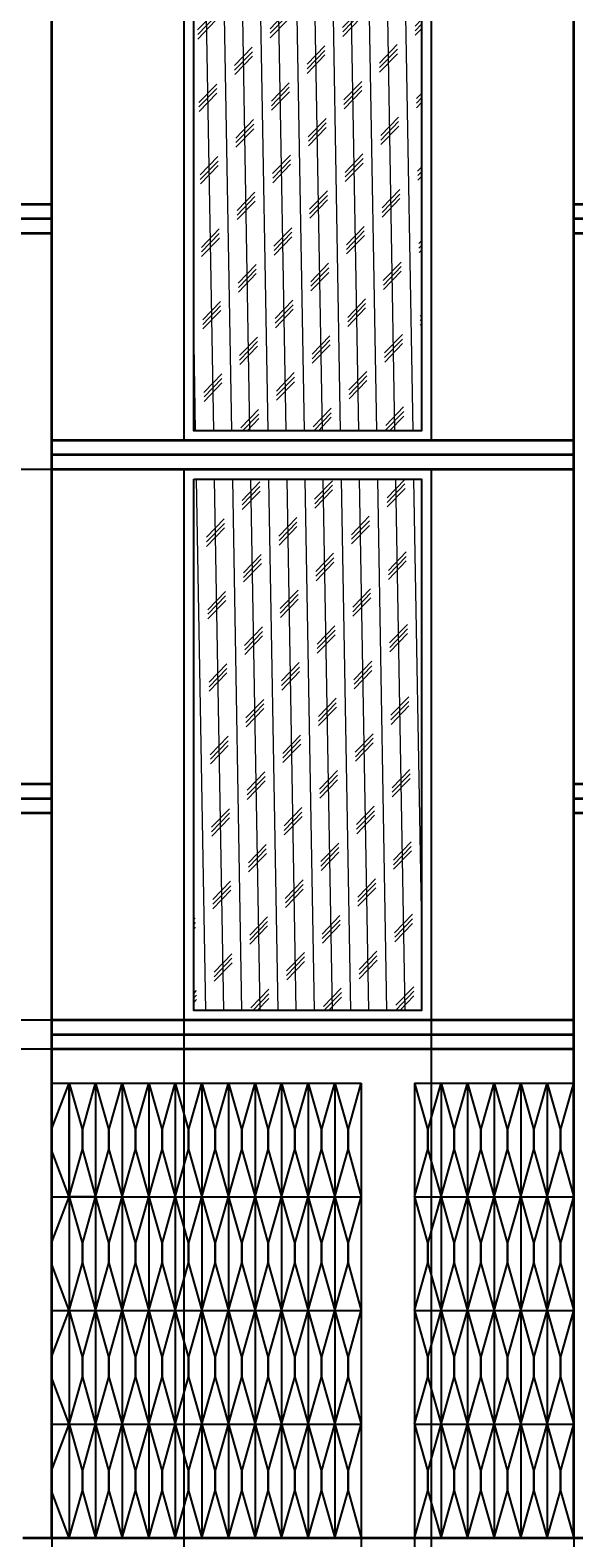
# Model space of a CAD drawing. Units: inches. Extents: x -742 to 1386, y -64 to 951.
# Tile 5 of 8: x 264 to 376, y 106 to 418. Entities that reach past the tile are written whole.
import ezdxf

# ---------------------------------------------------------------- set-up
doc = ezdxf.new("R2010")
doc.units = ezdxf.units.IN
doc.header["$MEASUREMENT"] = 0
for name, color, linetype, lineweight in [('A-ANNO-DIMS', 2, 'Continuous', 18), ('A-DOOR', 31, 'Continuous', 25), ('A-ELEV', 7, 'Continuous', 35), ('A-GLAZ', 4, 'Continuous', 25), ('A-GLAZ-PATT', 9, 'Continuous', 13)]:
    doc.layers.add(name, color=color, linetype=linetype, lineweight=lineweight)
doc.styles.get("Standard").update_dxf_attribs({"font": 'arial.ttf'})
doc.dimstyles.get("Standard").update_dxf_attribs({"dimtxt": 0.18, "dimasz": 0.18, "dimexe": 0.18, "dimexo": 0.0625, "dimgap": 0.09, "dimtad": 0, "dimtih": 1, "dimtoh": 1, "dimdec": 4, "dimzin": 0, "dimdsep": 46, "dimtxsty": 'Standard', "dimcen": 0.09, "dimadec": 0, "dimazin": 0, "dimtfac": 1, "dimtdec": 4, "dimtofl": 0, "dimtmove": 0, "dimatfit": 3, "dimfxl": 1, "dimtolj": 1, "dimtzin": 0, "dimarcsym": 0})
pattern_1 = [(91, (0, 0), (-3.74943, -0.065447), []), (226, (1.842, 1.907), (7.62975, -7.36796), [5.3033, -5.3033]), (226, (1.826, 2.845), (7.62975, -7.36796), [5.3033, -5.3033]), (226, (1.809, 3.782), (7.62975, -7.36796), [5.3033, -5.3033])]

# ---------------------------------------------------------------- blocks, each defined once
blk = doc.blocks.new('*D33')
at = {"layer": 'A-ANNO-DIMS', "color": 0, "lineweight": -2, "transparency": 16777216}
for p, q in [((268.23, 199.77), (268.23, -63.58)), ((332.25, 199.77), (332.25, -63.58)), ((268.41, -63.4), (299.84, -63.4)), ((332.07, -63.4), (300.63, -63.4))]:
    blk.add_line(p, q, dxfattribs=at)
at = {"layer": 'A-ANNO-DIMS', "color": 0, "transparency": 16777216}
for points in [[(268.41, -63.37), (268.41, -63.43), (268.23, -63.4)], [(332.07, -63.37), (332.07, -63.43), (332.25, -63.4)]]:
    blk.add_solid(points, dxfattribs=at)
at = {"layer": 'Defpoints', "color": 0, "transparency": 16777216}
for p in [(268.23, 199.83), (332.25, 199.83), (332.25, -63.4)]:
    blk.add_point(p, dxfattribs=at)
at = {"layer": 'A-ANNO-DIMS', "color": 0, "transparency": 16777216, "insert": (300.24, -63.4), "char_height": 0.18, "attachment_point": 5}
blk.add_mtext('\\A1;64.02', dxfattribs=at)
blk = doc.blocks.new('*D34')
at = {"layer": 'A-ANNO-DIMS', "color": 0, "lineweight": -2, "transparency": 16777216}
for p, q in [((332.25, 199.77), (332.25, -63.58)), ((343.24, 199.77), (343.24, -63.58)), ((332.43, -63.4), (337.29, -63.4)), ((343.06, -63.4), (338.2, -63.4))]:
    blk.add_line(p, q, dxfattribs=at)
at = {"layer": 'A-ANNO-DIMS', "color": 0, "transparency": 16777216}
for points in [[(332.43, -63.37), (332.43, -63.43), (332.25, -63.4)], [(343.06, -63.37), (343.06, -63.43), (343.24, -63.4)]]:
    blk.add_solid(points, dxfattribs=at)
at = {"layer": 'Defpoints', "color": 0, "transparency": 16777216}
for p in [(332.25, 199.83), (343.24, 199.83), (343.24, -63.4)]:
    blk.add_point(p, dxfattribs=at)
at = {"layer": 'A-ANNO-DIMS', "color": 0, "transparency": 16777216, "insert": (337.75, -63.4), "char_height": 0.18, "attachment_point": 5}
blk.add_mtext('\\A1;10.995', dxfattribs=at)
blk = doc.blocks.new('*D35')
at = {"layer": 'A-ANNO-DIMS', "color": 0, "lineweight": -2, "transparency": 16777216}
for p, q in [((343.24, 199.77), (343.24, -63.58)), ((376.23, 199.77), (376.23, -63.58)), ((343.42, -63.4), (359.27, -63.4)), ((376.05, -63.4), (360.2, -63.4))]:
    blk.add_line(p, q, dxfattribs=at)
at = {"layer": 'A-ANNO-DIMS', "color": 0, "transparency": 16777216}
for points in [[(343.42, -63.37), (343.42, -63.43), (343.24, -63.4)], [(376.05, -63.37), (376.05, -63.43), (376.23, -63.4)]]:
    blk.add_solid(points, dxfattribs=at)
at = {"layer": 'Defpoints', "color": 0, "transparency": 16777216}
for p in [(343.24, 199.83), (376.23, 199.83), (376.23, -63.4)]:
    blk.add_point(p, dxfattribs=at)
at = {"layer": 'A-ANNO-DIMS', "color": 0, "transparency": 16777216, "insert": (359.74, -63.4), "char_height": 0.18, "attachment_point": 5}
blk.add_mtext('\\A1;32.985', dxfattribs=at)
blk = doc.blocks.new('*D37')
at = {"layer": 'A-ANNO-DIMS', "color": 0, "lineweight": -2, "transparency": 16777216}
for p, q in [((268.23, 326.79), (268.23, -63.58)), ((295.56, 326.79), (295.56, -63.58)), ((268.41, -63.4), (281.43, -63.4)), ((295.38, -63.4), (282.36, -63.4))]:
    blk.add_line(p, q, dxfattribs=at)
at = {"layer": 'A-ANNO-DIMS', "color": 0, "transparency": 16777216}
for points in [[(268.41, -63.37), (268.41, -63.43), (268.23, -63.4)], [(295.38, -63.37), (295.38, -63.43), (295.56, -63.4)]]:
    blk.add_solid(points, dxfattribs=at)
at = {"layer": 'Defpoints', "color": 0, "transparency": 16777216}
for p in [(268.23, 326.85), (295.56, 326.85), (295.56, -63.4)]:
    blk.add_point(p, dxfattribs=at)
at = {"layer": 'A-ANNO-DIMS', "color": 0, "transparency": 16777216, "insert": (281.9, -63.4), "char_height": 0.18, "attachment_point": 5}
blk.add_mtext('\\A1;27.337', dxfattribs=at)
blk = doc.blocks.new('*D38')
at = {"layer": 'A-ANNO-DIMS', "color": 0, "lineweight": -2, "transparency": 16777216}
for p, q in [((295.56, 326.79), (295.56, -63.58)), ((346.7, 326.79), (346.7, -63.58)), ((295.74, -63.4), (320.74, -63.4)), ((346.52, -63.4), (321.52, -63.4))]:
    blk.add_line(p, q, dxfattribs=at)
at = {"layer": 'A-ANNO-DIMS', "color": 0, "transparency": 16777216}
for points in [[(295.74, -63.37), (295.74, -63.43), (295.56, -63.4)], [(346.52, -63.37), (346.52, -63.43), (346.7, -63.4)]]:
    blk.add_solid(points, dxfattribs=at)
at = {"layer": 'Defpoints', "color": 0, "transparency": 16777216}
for p in [(295.56, 326.85), (346.7, 326.85), (346.7, -63.4)]:
    blk.add_point(p, dxfattribs=at)
at = {"layer": 'A-ANNO-DIMS', "color": 0, "transparency": 16777216, "insert": (321.13, -63.4), "char_height": 0.18, "attachment_point": 5}
blk.add_mtext('\\A1;51.13', dxfattribs=at)
blk = doc.blocks.new('*D55')
at = {"layer": 'A-ANNO-DIMS', "color": 0, "lineweight": -2, "transparency": 16777216}
for p, q in [((295.5, 326.85), (-741.55, 326.85)), ((-741.37, 326.67), (-741.37, 270.04)), ((-741.37, 213.03), (-741.37, 269.67)), ((295.5, 212.85), (-741.55, 212.85))]:
    blk.add_line(p, q, dxfattribs=at)
at = {"layer": 'A-ANNO-DIMS', "color": 0, "transparency": 16777216}
for points in [[(-741.4, 326.67), (-741.34, 326.67), (-741.37, 326.85)], [(-741.4, 213.03), (-741.34, 213.03), (-741.37, 212.85)]]:
    blk.add_solid(points, dxfattribs=at)
at = {"layer": 'Defpoints', "color": 0, "transparency": 16777216}
for p in [(-741.37, 326.85), (295.56, 326.85), (295.56, 212.85)]:
    blk.add_point(p, dxfattribs=at)
at = {"layer": 'A-ANNO-DIMS', "color": 0, "transparency": 16777216, "insert": (-741.37, 269.85), "char_height": 0.18, "attachment_point": 5}
blk.add_mtext('\\A1;114', dxfattribs=at)
blk = doc.blocks.new('*D56')
at = {"layer": 'A-ANNO-DIMS', "color": 0, "lineweight": -2, "transparency": 16777216}
for p, q in [((268.17, 212.85), (-741.55, 212.85)), ((-741.37, 212.67), (-741.37, 210.04)), ((-741.37, 207.03), (-741.37, 209.67)), ((268.17, 206.85), (-741.55, 206.85))]:
    blk.add_line(p, q, dxfattribs=at)
at = {"layer": 'A-ANNO-DIMS', "color": 0, "transparency": 16777216}
for points in [[(-741.4, 212.67), (-741.34, 212.67), (-741.37, 212.85)], [(-741.4, 207.03), (-741.34, 207.03), (-741.37, 206.85)]]:
    blk.add_solid(points, dxfattribs=at)
at = {"layer": 'Defpoints', "color": 0, "transparency": 16777216}
for p in [(-741.37, 212.85), (268.23, 212.85), (268.23, 206.85)]:
    blk.add_point(p, dxfattribs=at)
at = {"layer": 'A-ANNO-DIMS', "color": 0, "transparency": 16777216, "insert": (-741.37, 209.85), "char_height": 0.18, "attachment_point": 5}
blk.add_mtext('\\A1;6', dxfattribs=at)

msp = doc.modelspace()

# ---------------------------------------------------------------- hatches: boundary and pattern name
at = {"layer": 'A-GLAZ-PATT', "transparency": 33554457}
h = msp.add_hatch(dxfattribs=at)
h.set_pattern_fill('CORK', color=256, scale=30, angle=91)
h.set_pattern_definition(pattern_1)
h.paths.add_polyline_path([(344.6973, 444.8548), (297.5643, 444.8548), (297.5643, 334.8548), (344.6973, 334.8548)])
h = msp.add_hatch(dxfattribs=at)
h.set_pattern_fill('CORK', color=256, scale=30, angle=91)
h.set_pattern_definition(pattern_1)
h.paths.add_polyline_path([(344.6973, 324.8548), (297.5643, 324.8548), (297.5643, 214.8548), (344.6973, 214.8548)])

# ---------------------------------------------------------------- linework, layer by layer
at = {"layer": 'A-DOOR'}
for p, q in [((268.2276, 199.8339), (332.2479, 199.8339)), ((268.2276, 190.4167), (271.776, 199.8339)), ((271.776, 199.8339), (271.776, 105.7399)), ((271.776, 199.8339), (274.5247, 190.0721)), ((274.5247, 190.0721), (277.2734, 199.8339)), ((277.2734, 199.8339), (277.2734, 105.7399)), ((277.2734, 199.8339), (280.0221, 190.0721)), ((280.0221, 190.0721), (282.7709, 199.8339)), ((282.7709, 199.8339), (282.7709, 105.7399)), ((282.7709, 199.8339), (285.5196, 190.0721)), ((285.5196, 190.0721), (288.2683, 199.8339)), ((288.2683, 199.8339), (288.2683, 105.7399)), ((288.2683, 199.8339), (291.017, 190.0721)), ((291.017, 190.0721), (293.7658, 199.8339)), ((293.7658, 199.8339), (293.7658, 105.7399)), ((293.7658, 199.8339), (296.5145, 190.0721)), ((296.5145, 190.0721), (299.2632, 199.8339)), ((299.2632, 199.8339), (299.2632, 105.7399)), ((299.2632, 199.8339), (302.012, 190.0721)), ((302.012, 190.0721), (304.7607, 199.8339)), ((304.7607, 199.8339), (304.7607, 105.7399)), ((304.7607, 199.8339), (307.5094, 190.0721)), ((307.5094, 190.0721), (310.2581, 199.8339)), ((310.2581, 199.8339), (310.2581, 105.7399)), ((310.2581, 199.8339), (313.0069, 190.0721)), ((313.0069, 190.0721), (315.7556, 199.8339)), ((315.7556, 199.8339), (315.7556, 105.7399)), ((315.7556, 199.8339), (318.5043, 190.0721)), ((318.5043, 190.0721), (321.253, 199.8339)), ((321.253, 199.8339), (321.253, 105.7399)), ((321.253, 199.8339), (324.0018, 190.0721)), ((324.0018, 190.0721), (326.7505, 199.8339)), ((326.7505, 199.8339), (326.7505, 105.7399)), ((326.7505, 199.8339), (329.4992, 190.0721)), ((329.4992, 190.0721), (332.2479, 199.8339)), ((332.2479, 199.8339), (332.2479, 105.7399)), ((343.2429, 199.8339), (343.2429, 105.7399)), ((343.2429, 199.8339), (345.9916, 190.0721)), ((343.2429, 199.8339), (376.2276, 199.8339)), ((345.9916, 190.0721), (348.7403, 199.8339)), ((348.7403, 199.8339), (348.7403, 105.7399)), ((348.7403, 199.8339), (351.489, 190.0721)), ((351.489, 190.0721), (354.2378, 199.8339)), ((354.2378, 199.8339), (354.2378, 105.7399)), ((354.2378, 199.8339), (356.9865, 190.0721)), ((356.9865, 190.0721), (359.7352, 199.8339)), ((359.7352, 199.8339), (359.7352, 105.7399)), ((359.7352, 199.8339), (362.4839, 190.0721)), ((362.4839, 190.0721), (365.2327, 199.8339)), ((365.2327, 199.8339), (365.2327, 105.7399)), ((365.2327, 199.8339), (367.9814, 190.0721)), ((367.9814, 190.0721), (370.7301, 199.8339)), ((370.7301, 199.8339), (370.7301, 105.7399)), ((370.7301, 199.8339), (373.4788, 190.0721)), ((373.4788, 190.0721), (376.2276, 199.8339)), ((376.2276, 199.8339), (376.2276, 105.7399)), ((274.5247, 186.0721), (274.5247, 190.0721)), ((274.5247, 190.0721), (274.5247, 186.0721)), ((280.0221, 186.0721), (280.0221, 190.0721)), ((280.0221, 190.0721), (280.0221, 186.0721)), ((285.5196, 186.0721), (285.5196, 190.0721)), ((285.5196, 190.0721), (285.5196, 186.0721)), ((291.017, 186.0721), (291.017, 190.0721)), ((291.017, 190.0721), (291.017, 186.0721)), ((296.5145, 186.0721), (296.5145, 190.0721)), ((296.5145, 190.0721), (296.5145, 186.0721)), ((302.012, 186.0721), (302.012, 190.0721)), ((302.012, 190.0721), (302.012, 186.0721)), ((307.5094, 186.0721), (307.5094, 190.0721)), ((307.5094, 190.0721), (307.5094, 186.0721)), ((313.0069, 186.0721), (313.0069, 190.0721)), ((313.0069, 190.0721), (313.0069, 186.0721)), ((318.5043, 186.0721), (318.5043, 190.0721)), ((318.5043, 190.0721), (318.5043, 186.0721)), ((324.0018, 186.0721), (324.0018, 190.0721)), ((324.0018, 190.0721), (324.0018, 186.0721)), ((329.4992, 186.0721), (329.4992, 190.0721)), ((329.4992, 190.0721), (329.4992, 186.0721)), ((345.9916, 186.0721), (345.9916, 190.0721)), ((345.9916, 190.0721), (345.9916, 186.0721)), ((351.489, 186.0721), (351.489, 190.0721)), ((351.489, 190.0721), (351.489, 186.0721)), ((356.9865, 186.0721), (356.9865, 190.0721)), ((356.9865, 190.0721), (356.9865, 186.0721)), ((362.4839, 186.0721), (362.4839, 190.0721)), ((362.4839, 190.0721), (362.4839, 186.0721)), ((367.9814, 186.0721), (367.9814, 190.0721)), ((367.9814, 190.0721), (367.9814, 186.0721)), ((373.4788, 186.0721), (373.4788, 190.0721)), ((373.4788, 190.0721), (373.4788, 186.0721)), ((271.776, 176.3104), (268.2276, 185.8171)), ((271.776, 176.3104), (274.5247, 186.0721)), ((274.5247, 186.0721), (277.2734, 176.3104)), ((277.2734, 176.3104), (280.0221, 186.0721)), ((280.0221, 186.0721), (282.7709, 176.3104)), ((282.7709, 176.3104), (285.5196, 186.0721)), ((285.5196, 186.0721), (288.2683, 176.3104)), ((288.2683, 176.3104), (291.017, 186.0721)), ((291.017, 186.0721), (293.7658, 176.3104)), ((293.7658, 176.3104), (296.5145, 186.0721)), ((296.5145, 186.0721), (299.2632, 176.3104)), ((299.2632, 176.3104), (302.012, 186.0721)), ((302.012, 186.0721), (304.7607, 176.3104)), ((304.7607, 176.3104), (307.5094, 186.0721)), ((307.5094, 186.0721), (310.2581, 176.3104)), ((310.2581, 176.3104), (313.0069, 186.0721)), ((313.0069, 186.0721), (315.7556, 176.3104)), ((315.7556, 176.3104), (318.5043, 186.0721)), ((318.5043, 186.0721), (321.253, 176.3104)), ((321.253, 176.3104), (324.0018, 186.0721)), ((324.0018, 186.0721), (326.7505, 176.3104)), ((326.7505, 176.3104), (329.4992, 186.0721)), ((329.4992, 186.0721), (332.2479, 176.3104)), ((343.2429, 176.3104), (345.9916, 186.0721)), ((345.9916, 186.0721), (348.7403, 176.3104)), ((348.7403, 176.3104), (351.489, 186.0721)), ((351.489, 186.0721), (354.2378, 176.3104)), ((354.2378, 176.3104), (356.9865, 186.0721)), ((356.9865, 186.0721), (359.7352, 176.3104)), ((359.7352, 176.3104), (362.4839, 186.0721)), ((362.4839, 186.0721), (365.2327, 176.3104)), ((365.2327, 176.3104), (367.9814, 186.0721)), ((367.9814, 186.0721), (370.7301, 176.3104)), ((370.7301, 176.3104), (373.4788, 186.0721)), ((373.4788, 186.0721), (376.2276, 176.3104)), ((268.2276, 176.3104), (332.2479, 176.3104)), ((268.2276, 166.8932), (271.776, 176.3104)), ((271.776, 176.3104), (274.5247, 166.5486)), ((274.5247, 166.5486), (277.2734, 176.3104)), ((277.2734, 176.3104), (280.0221, 166.5486)), ((280.0221, 166.5486), (282.7709, 176.3104)), ((282.7709, 176.3104), (285.5196, 166.5486)), ((285.5196, 166.5486), (288.2683, 176.3104)), ((288.2683, 176.3104), (291.017, 166.5486)), ((291.017, 166.5486), (293.7658, 176.3104)), ((293.7658, 176.3104), (296.5145, 166.5486)), ((296.5145, 166.5486), (299.2632, 176.3104)), ((299.2632, 176.3104), (302.012, 166.5486)), ((302.012, 166.5486), (304.7607, 176.3104)), ((304.7607, 176.3104), (307.5094, 166.5486)), ((307.5094, 166.5486), (310.2581, 176.3104)), ((310.2581, 176.3104), (313.0069, 166.5486)), ((313.0069, 166.5486), (315.7556, 176.3104)), ((315.7556, 176.3104), (318.5043, 166.5486)), ((318.5043, 166.5486), (321.253, 176.3104)), ((321.253, 176.3104), (324.0018, 166.5486)), ((324.0018, 166.5486), (326.7505, 176.3104)), ((326.7505, 176.3104), (329.4992, 166.5486)), ((329.4992, 166.5486), (332.2479, 176.3104)), ((343.2429, 176.3104), (345.9916, 166.5486)), ((343.2429, 176.3104), (376.2276, 176.3104)), ((345.9916, 166.5486), (348.7403, 176.3104)), ((348.7403, 176.3104), (351.489, 166.5486)), ((351.489, 166.5486), (354.2378, 176.3104)), ((354.2378, 176.3104), (356.9865, 166.5486)), ((356.9865, 166.5486), (359.7352, 176.3104)), ((359.7352, 176.3104), (362.4839, 166.5486)), ((362.4839, 166.5486), (365.2327, 176.3104)), ((365.2327, 176.3104), (367.9814, 166.5486)), ((367.9814, 166.5486), (370.7301, 176.3104)), ((370.7301, 176.3104), (373.4788, 166.5486)), ((373.4788, 166.5486), (376.2276, 176.3104)), ((274.5247, 162.5486), (274.5247, 166.5486)), ((274.5247, 166.5486), (274.5247, 162.5486)), ((280.0221, 162.5486), (280.0221, 166.5486)), ((280.0221, 166.5486), (280.0221, 162.5486)), ((285.5196, 162.5486), (285.5196, 166.5486)), ((285.5196, 166.5486), (285.5196, 162.5486)), ((291.017, 162.5486), (291.017, 166.5486)), ((291.017, 166.5486), (291.017, 162.5486)), ((296.5145, 162.5486), (296.5145, 166.5486)), ((296.5145, 166.5486), (296.5145, 162.5486)), ((302.012, 162.5486), (302.012, 166.5486)), ((302.012, 166.5486), (302.012, 162.5486)), ((307.5094, 162.5486), (307.5094, 166.5486)), ((307.5094, 166.5486), (307.5094, 162.5486)), ((313.0069, 162.5486), (313.0069, 166.5486)), ((313.0069, 166.5486), (313.0069, 162.5486)), ((318.5043, 162.5486), (318.5043, 166.5486)), ((318.5043, 166.5486), (318.5043, 162.5486)), ((324.0018, 162.5486), (324.0018, 166.5486)), ((324.0018, 166.5486), (324.0018, 162.5486)), ((329.4992, 162.5486), (329.4992, 166.5486)), ((329.4992, 166.5486), (329.4992, 162.5486)), ((345.9916, 162.5486), (345.9916, 166.5486)), ((345.9916, 166.5486), (345.9916, 162.5486)), ((351.489, 162.5486), (351.489, 166.5486)), ((351.489, 166.5486), (351.489, 162.5486)), ((356.9865, 162.5486), (356.9865, 166.5486)), ((356.9865, 166.5486), (356.9865, 162.5486)), ((362.4839, 162.5486), (362.4839, 166.5486)), ((362.4839, 166.5486), (362.4839, 162.5486)), ((367.9814, 162.5486), (367.9814, 166.5486)), ((367.9814, 166.5486), (367.9814, 162.5486)), ((373.4788, 162.5486), (373.4788, 166.5486)), ((373.4788, 166.5486), (373.4788, 162.5486)), ((271.776, 152.7869), (268.2276, 162.2936)), ((271.776, 152.7869), (274.5247, 162.5486)), ((274.5247, 162.5486), (277.2734, 152.7869)), ((277.2734, 152.7869), (280.0221, 162.5486)), ((280.0221, 162.5486), (282.7709, 152.7869)), ((282.7709, 152.7869), (285.5196, 162.5486)), ((285.5196, 162.5486), (288.2683, 152.7869)), ((288.2683, 152.7869), (291.017, 162.5486)), ((291.017, 162.5486), (293.7658, 152.7869)), ((293.7658, 152.7869), (296.5145, 162.5486)), ((296.5145, 162.5486), (299.2632, 152.7869)), ((299.2632, 152.7869), (302.012, 162.5486)), ((302.012, 162.5486), (304.7607, 152.7869)), ((304.7607, 152.7869), (307.5094, 162.5486)), ((307.5094, 162.5486), (310.2581, 152.7869)), ((310.2581, 152.7869), (313.0069, 162.5486)), ((313.0069, 162.5486), (315.7556, 152.7869)), ((315.7556, 152.7869), (318.5043, 162.5486)), ((318.5043, 162.5486), (321.253, 152.7869)), ((321.253, 152.7869), (324.0018, 162.5486)), ((324.0018, 162.5486), (326.7505, 152.7869)), ((326.7505, 152.7869), (329.4992, 162.5486)), ((329.4992, 162.5486), (332.2479, 152.7869)), ((343.2429, 152.7869), (345.9916, 162.5486)), ((345.9916, 162.5486), (348.7403, 152.7869)), ((348.7403, 152.7869), (351.489, 162.5486)), ((351.489, 162.5486), (354.2378, 152.7869)), ((354.2378, 152.7869), (356.9865, 162.5486)), ((356.9865, 162.5486), (359.7352, 152.7869)), ((359.7352, 152.7869), (362.4839, 162.5486)), ((362.4839, 162.5486), (365.2327, 152.7869)), ((365.2327, 152.7869), (367.9814, 162.5486)), ((367.9814, 162.5486), (370.7301, 152.7869)), ((370.7301, 152.7869), (373.4788, 162.5486)), ((373.4788, 162.5486), (376.2276, 152.7869)), ((268.2276, 152.7869), (332.2479, 152.7869)), ((268.2276, 143.3697), (271.776, 152.7869)), ((271.776, 152.7869), (274.5247, 143.0251)), ((274.5247, 143.0251), (277.2734, 152.7869)), ((277.2734, 152.7869), (280.0221, 143.0251)), ((280.0221, 143.0251), (282.7709, 152.7869)), ((282.7709, 152.7869), (285.5196, 143.0251)), ((285.5196, 143.0251), (288.2683, 152.7869)), ((288.2683, 152.7869), (291.017, 143.0251)), ((291.017, 143.0251), (293.7658, 152.7869)), ((293.7658, 152.7869), (296.5145, 143.0251)), ((296.5145, 143.0251), (299.2632, 152.7869)), ((299.2632, 152.7869), (302.012, 143.0251)), ((302.012, 143.0251), (304.7607, 152.7869)), ((304.7607, 152.7869), (307.5094, 143.0251)), ((307.5094, 143.0251), (310.2581, 152.7869)), ((310.2581, 152.7869), (313.0069, 143.0251)), ((313.0069, 143.0251), (315.7556, 152.7869)), ((315.7556, 152.7869), (318.5043, 143.0251)), ((318.5043, 143.0251), (321.253, 152.7869)), ((321.253, 152.7869), (324.0018, 143.0251)), ((324.0018, 143.0251), (326.7505, 152.7869)), ((326.7505, 152.7869), (329.4992, 143.0251)), ((329.4992, 143.0251), (332.2479, 152.7869)), ((343.2429, 152.7869), (345.9916, 143.0251)), ((343.2429, 152.7869), (376.2276, 152.7869)), ((345.9916, 143.0251), (348.7403, 152.7869)), ((348.7403, 152.7869), (351.489, 143.0251)), ((351.489, 143.0251), (354.2378, 152.7869)), ((354.2378, 152.7869), (356.9865, 143.0251)), ((356.9865, 143.0251), (359.7352, 152.7869)), ((359.7352, 152.7869), (362.4839, 143.0251)), ((362.4839, 143.0251), (365.2327, 152.7869)), ((365.2327, 152.7869), (367.9814, 143.0251)), ((367.9814, 143.0251), (370.7301, 152.7869)), ((370.7301, 152.7869), (373.4788, 143.0251)), ((373.4788, 143.0251), (376.2276, 152.7869)), ((274.5247, 139.0251), (274.5247, 143.0251)), ((274.5247, 143.0251), (274.5247, 139.0251)), ((280.0221, 139.0251), (280.0221, 143.0251)), ((280.0221, 143.0251), (280.0221, 139.0251)), ((285.5196, 139.0251), (285.5196, 143.0251)), ((285.5196, 143.0251), (285.5196, 139.0251)), ((291.017, 139.0251), (291.017, 143.0251)), ((291.017, 143.0251), (291.017, 139.0251)), ((296.5145, 139.0251), (296.5145, 143.0251)), ((296.5145, 143.0251), (296.5145, 139.0251)), ((302.012, 139.0251), (302.012, 143.0251)), ((302.012, 143.0251), (302.012, 139.0251)), ((307.5094, 139.0251), (307.5094, 143.0251)), ((307.5094, 143.0251), (307.5094, 139.0251)), ((313.0069, 139.0251), (313.0069, 143.0251)), ((313.0069, 143.0251), (313.0069, 139.0251)), ((318.5043, 139.0251), (318.5043, 143.0251)), ((318.5043, 143.0251), (318.5043, 139.0251)), ((324.0018, 139.0251), (324.0018, 143.0251)), ((324.0018, 143.0251), (324.0018, 139.0251)), ((329.4992, 139.0251), (329.4992, 143.0251)), ((329.4992, 143.0251), (329.4992, 139.0251)), ((345.9916, 139.0251), (345.9916, 143.0251)), ((345.9916, 143.0251), (345.9916, 139.0251)), ((351.489, 139.0251), (351.489, 143.0251)), ((351.489, 143.0251), (351.489, 139.0251)), ((356.9865, 139.0251), (356.9865, 143.0251)), ((356.9865, 143.0251), (356.9865, 139.0251)), ((362.4839, 139.0251), (362.4839, 143.0251)), ((362.4839, 143.0251), (362.4839, 139.0251)), ((367.9814, 139.0251), (367.9814, 143.0251)), ((367.9814, 143.0251), (367.9814, 139.0251)), ((373.4788, 139.0251), (373.4788, 143.0251)), ((373.4788, 143.0251), (373.4788, 139.0251)), ((271.776, 129.2634), (268.2276, 138.7701)), ((271.776, 129.2634), (274.5247, 139.0251)), ((274.5247, 139.0251), (277.2734, 129.2634)), ((277.2734, 129.2634), (280.0221, 139.0251)), ((280.0221, 139.0251), (282.7709, 129.2634)), ((282.7709, 129.2634), (285.5196, 139.0251)), ((285.5196, 139.0251), (288.2683, 129.2634)), ((288.2683, 129.2634), (291.017, 139.0251)), ((291.017, 139.0251), (293.7658, 129.2634)), ((293.7658, 129.2634), (296.5145, 139.0251)), ((296.5145, 139.0251), (299.2632, 129.2634)), ((299.2632, 129.2634), (302.012, 139.0251)), ((302.012, 139.0251), (304.7607, 129.2634)), ((304.7607, 129.2634), (307.5094, 139.0251)), ((307.5094, 139.0251), (310.2581, 129.2634)), ((310.2581, 129.2634), (313.0069, 139.0251)), ((313.0069, 139.0251), (315.7556, 129.2634)), ((315.7556, 129.2634), (318.5043, 139.0251)), ((318.5043, 139.0251), (321.253, 129.2634)), ((321.253, 129.2634), (324.0018, 139.0251)), ((324.0018, 139.0251), (326.7505, 129.2634)), ((326.7505, 129.2634), (329.4992, 139.0251)), ((329.4992, 139.0251), (332.2479, 129.2634)), ((343.2429, 129.2634), (345.9916, 139.0251)), ((345.9916, 139.0251), (348.7403, 129.2634)), ((348.7403, 129.2634), (351.489, 139.0251)), ((351.489, 139.0251), (354.2378, 129.2634)), ((354.2378, 129.2634), (356.9865, 139.0251)), ((356.9865, 139.0251), (359.7352, 129.2634)), ((359.7352, 129.2634), (362.4839, 139.0251)), ((362.4839, 139.0251), (365.2327, 129.2634)), ((365.2327, 129.2634), (367.9814, 139.0251)), ((367.9814, 139.0251), (370.7301, 129.2634)), ((370.7301, 129.2634), (373.4788, 139.0251)), ((373.4788, 139.0251), (376.2276, 129.2634)), ((268.2276, 129.2634), (332.2479, 129.2634)), ((268.2276, 119.8462), (271.776, 129.2634)), ((271.776, 129.2634), (274.5247, 119.5016)), ((274.5247, 119.5016), (277.2734, 129.2634)), ((277.2734, 129.2634), (280.0221, 119.5016)), ((280.0221, 119.5016), (282.7709, 129.2634)), ((282.7709, 129.2634), (285.5196, 119.5016)), ((285.5196, 119.5016), (288.2683, 129.2634)), ((288.2683, 129.2634), (291.017, 119.5016)), ((291.017, 119.5016), (293.7658, 129.2634)), ((293.7658, 129.2634), (296.5145, 119.5016)), ((296.5145, 119.5016), (299.2632, 129.2634)), ((299.2632, 129.2634), (302.012, 119.5016)), ((302.012, 119.5016), (304.7607, 129.2634)), ((304.7607, 129.2634), (307.5094, 119.5016)), ((307.5094, 119.5016), (310.2581, 129.2634)), ((310.2581, 129.2634), (313.0069, 119.5016)), ((313.0069, 119.5016), (315.7556, 129.2634)), ((315.7556, 129.2634), (318.5043, 119.5016)), ((318.5043, 119.5016), (321.253, 129.2634)), ((321.253, 129.2634), (324.0018, 119.5016)), ((324.0018, 119.5016), (326.7505, 129.2634)), ((326.7505, 129.2634), (329.4992, 119.5016)), ((329.4992, 119.5016), (332.2479, 129.2634)), ((343.2429, 129.2634), (345.9916, 119.5016)), ((343.2429, 129.2634), (376.2276, 129.2634)), ((345.9916, 119.5016), (348.7403, 129.2634)), ((348.7403, 129.2634), (351.489, 119.5016)), ((351.489, 119.5016), (354.2378, 129.2634)), ((354.2378, 129.2634), (356.9865, 119.5016)), ((356.9865, 119.5016), (359.7352, 129.2634)), ((359.7352, 129.2634), (362.4839, 119.5016)), ((362.4839, 119.5016), (365.2327, 129.2634)), ((365.2327, 129.2634), (367.9814, 119.5016)), ((367.9814, 119.5016), (370.7301, 129.2634)), ((370.7301, 129.2634), (373.4788, 119.5016)), ((373.4788, 119.5016), (376.2276, 129.2634)), ((274.5247, 115.5016), (274.5247, 119.5016)), ((274.5247, 119.5016), (274.5247, 115.5016)), ((280.0221, 115.5016), (280.0221, 119.5016)), ((280.0221, 119.5016), (280.0221, 115.5016)), ((285.5196, 115.5016), (285.5196, 119.5016)), ((285.5196, 119.5016), (285.5196, 115.5016)), ((291.017, 115.5016), (291.017, 119.5016)), ((291.017, 119.5016), (291.017, 115.5016)), ((296.5145, 115.5016), (296.5145, 119.5016)), ((296.5145, 119.5016), (296.5145, 115.5016)), ((302.012, 115.5016), (302.012, 119.5016)), ((302.012, 119.5016), (302.012, 115.5016)), ((307.5094, 115.5016), (307.5094, 119.5016)), ((307.5094, 119.5016), (307.5094, 115.5016)), ((313.0069, 115.5016), (313.0069, 119.5016)), ((313.0069, 119.5016), (313.0069, 115.5016)), ((318.5043, 115.5016), (318.5043, 119.5016)), ((318.5043, 119.5016), (318.5043, 115.5016)), ((324.0018, 115.5016), (324.0018, 119.5016)), ((324.0018, 119.5016), (324.0018, 115.5016)), ((329.4992, 115.5016), (329.4992, 119.5016)), ((329.4992, 119.5016), (329.4992, 115.5016)), ((345.9916, 115.5016), (345.9916, 119.5016)), ((345.9916, 119.5016), (345.9916, 115.5016)), ((351.489, 115.5016), (351.489, 119.5016)), ((351.489, 119.5016), (351.489, 115.5016)), ((356.9865, 115.5016), (356.9865, 119.5016)), ((356.9865, 119.5016), (356.9865, 115.5016)), ((362.4839, 115.5016), (362.4839, 119.5016)), ((362.4839, 119.5016), (362.4839, 115.5016)), ((367.9814, 115.5016), (367.9814, 119.5016)), ((367.9814, 119.5016), (367.9814, 115.5016)), ((373.4788, 115.5016), (373.4788, 119.5016)), ((373.4788, 119.5016), (373.4788, 115.5016)), ((271.776, 105.7399), (274.5247, 115.5016)), ((274.5247, 115.5016), (277.2734, 105.7399)), ((277.2734, 105.7399), (280.0221, 115.5016)), ((280.0221, 115.5016), (282.7709, 105.7399)), ((282.7709, 105.7399), (285.5196, 115.5016)), ((285.5196, 115.5016), (288.2683, 105.7399)), ((288.2683, 105.7399), (291.017, 115.5016)), ((291.017, 115.5016), (293.7658, 105.7399)), ((293.7658, 105.7399), (296.5145, 115.5016)), ((296.5145, 115.5016), (299.2632, 105.7399)), ((299.2632, 105.7399), (302.012, 115.5016)), ((302.012, 115.5016), (304.7607, 105.7399)), ((304.7607, 105.7399), (307.5094, 115.5016)), ((307.5094, 115.5016), (310.2581, 105.7399)), ((310.2581, 105.7399), (313.0069, 115.5016)), ((313.0069, 115.5016), (315.7556, 105.7399)), ((315.7556, 105.7399), (318.5043, 115.5016)), ((318.5043, 115.5016), (321.253, 105.7399)), ((321.253, 105.7399), (324.0018, 115.5016)), ((324.0018, 115.5016), (326.7505, 105.7399)), ((326.7505, 105.7399), (329.4992, 115.5016)), ((329.4992, 115.5016), (332.2479, 105.7399)), ((343.2429, 105.7399), (345.9916, 115.5016)), ((345.9916, 115.5016), (348.7403, 105.7399)), ((348.7403, 105.7399), (351.489, 115.5016)), ((351.489, 115.5016), (354.2378, 105.7399)), ((354.2378, 105.7399), (356.9865, 115.5016)), ((356.9865, 115.5016), (359.7352, 105.7399)), ((359.7352, 105.7399), (362.4839, 115.5016)), ((362.4839, 115.5016), (365.2327, 105.7399)), ((365.2327, 105.7399), (367.9814, 115.5016)), ((367.9814, 115.5016), (370.7301, 105.7399)), ((370.7301, 105.7399), (373.4788, 115.5016)), ((373.4788, 115.5016), (376.2276, 105.7399)), ((271.776, 105.7399), (268.2276, 115.2466)), ((268.2276, 105.7399), (376.2276, 105.7399))]:
    msp.add_line(p, q, dxfattribs=at)
msp.add_lwpolyline([(271.776, 199.8339), (277.2734, 199.8339), (277.2734, 176.3104), (271.776, 176.3104)], close=True, dxfattribs=at)
at = {"layer": 'A-ELEV'}
for p, q in [((268.2276, 105.7399), (268.2276, 835.7799)), ((376.2276, 105.7399), (376.2276, 835.7799)), ((-37.7724, 381.7399), (268.2276, 381.7399)), ((376.2276, 381.7399), (682.2276, 381.7399)), ((-37.7724, 378.7399), (268.2276, 378.7399)), ((376.2276, 378.7399), (682.2276, 378.7399)), ((-37.7724, 375.7399), (268.2276, 375.7399)), ((376.2276, 375.7399), (682.2276, 375.7399)), ((376.2276, 332.8548), (268.2276, 332.8548)), ((376.2276, 329.8548), (268.2276, 329.8548)), ((376.2276, 326.8548), (268.2276, 326.8548)), ((-37.7724, 261.7399), (268.2276, 261.7399)), ((376.2276, 261.7399), (622.2276, 261.7399)), ((-37.7724, 258.7399), (268.2276, 258.7399)), ((376.2276, 258.7399), (622.2276, 258.7399)), ((-37.7724, 255.7399), (268.2276, 255.7399)), ((376.2276, 255.7399), (622.2276, 255.7399)), ((376.2276, 212.8548), (268.2276, 212.8548)), ((376.2276, 209.8548), (268.2276, 209.8548)), ((376.2276, 206.8548), (268.2276, 206.8548)), ((262.2276, 105.7399), (682.2276, 105.7399))]:
    msp.add_line(p, q, dxfattribs=at)
at = {"layer": 'A-GLAZ'}
for points in [[(295.5643, 446.8548), (346.6973, 446.8548), (346.6973, 332.8548), (295.5643, 332.8548)], [(297.5643, 444.8548), (344.6973, 444.8548), (344.6973, 334.8548), (297.5643, 334.8548)], [(295.5643, 326.8548), (346.6973, 326.8548), (346.6973, 212.8548), (295.5643, 212.8548)], [(297.5643, 324.8548), (344.6973, 324.8548), (344.6973, 214.8548), (297.5643, 214.8548)]]:
    msp.add_lwpolyline(points, close=True, dxfattribs=at)

# ---------------------------------------------------------------- dimensions: what is measured, and where the dimension line sits
at = {"layer": 'A-ANNO-DIMS'}
for base, p1, p2, picture, middle in [((-741.3711, 326.8548), (295.5643, 212.8548), (295.5643, 326.8548), '*D55', (-741.3711, 269.8548)), ((-741.3711, 212.8548), (268.2276, 206.8548), (268.2276, 212.8548), '*D56', (-741.3711, 209.8548))]:
    dim = msp.add_linear_dim(base=base, p1=p1, p2=p2, angle=90, dimstyle='Standard', override={"dimdec": 0, "dimlfac": 1, "dimrnd": 0, "dimzin": 0, "dimdsep": 46, "dimlunit": 2}, dxfattribs=at)
    dim.commit()
    dim.dimension.update_dxf_attribs({"geometry": picture, "text_midpoint": middle})
for base, p1, p2, override, picture, middle in [((295.5643, -63.3971), (268.2276, 326.8548), (295.5643, 326.8548), {"dimdec": 3, "dimlfac": 1, "dimrnd": 0, "dimzin": 0, "dimdsep": 46, "dimlunit": 2}, '*D37', (281.896, -63.3971)), ((346.6973, -63.3971), (295.5643, 326.8548), (346.6973, 326.8548), {"dimdec": 2, "dimlfac": 1, "dimrnd": 0, "dimzin": 0, "dimdsep": 46, "dimlunit": 2}, '*D38', (321.1308, -63.3971)), ((332.2479, -63.3971), (268.2276, 199.8339), (332.2479, 199.8339), {"dimdec": 2, "dimlfac": 1, "dimrnd": 0, "dimzin": 0, "dimdsep": 46, "dimlunit": 2}, '*D33', (300.2378, -63.3971)), ((343.2429, -63.3971), (332.2479, 199.8339), (343.2429, 199.8339), {"dimdec": 3, "dimlfac": 1, "dimrnd": 0, "dimzin": 0, "dimdsep": 46, "dimlunit": 2}, '*D34', (337.7454, -63.3971)), ((376.2276, -63.3971), (343.2429, 199.8339), (376.2276, 199.8339), {"dimdec": 3, "dimlfac": 1, "dimrnd": 0, "dimzin": 0, "dimdsep": 46, "dimlunit": 2}, '*D35', (359.7352, -63.3971))]:
    dim = msp.add_linear_dim(base=base, p1=p1, p2=p2, dimstyle='Standard', override=override, dxfattribs=at)
    dim.commit()
    dim.dimension.update_dxf_attribs({"geometry": picture, "text_midpoint": middle})

doc.saveas('drawing.dxf')
